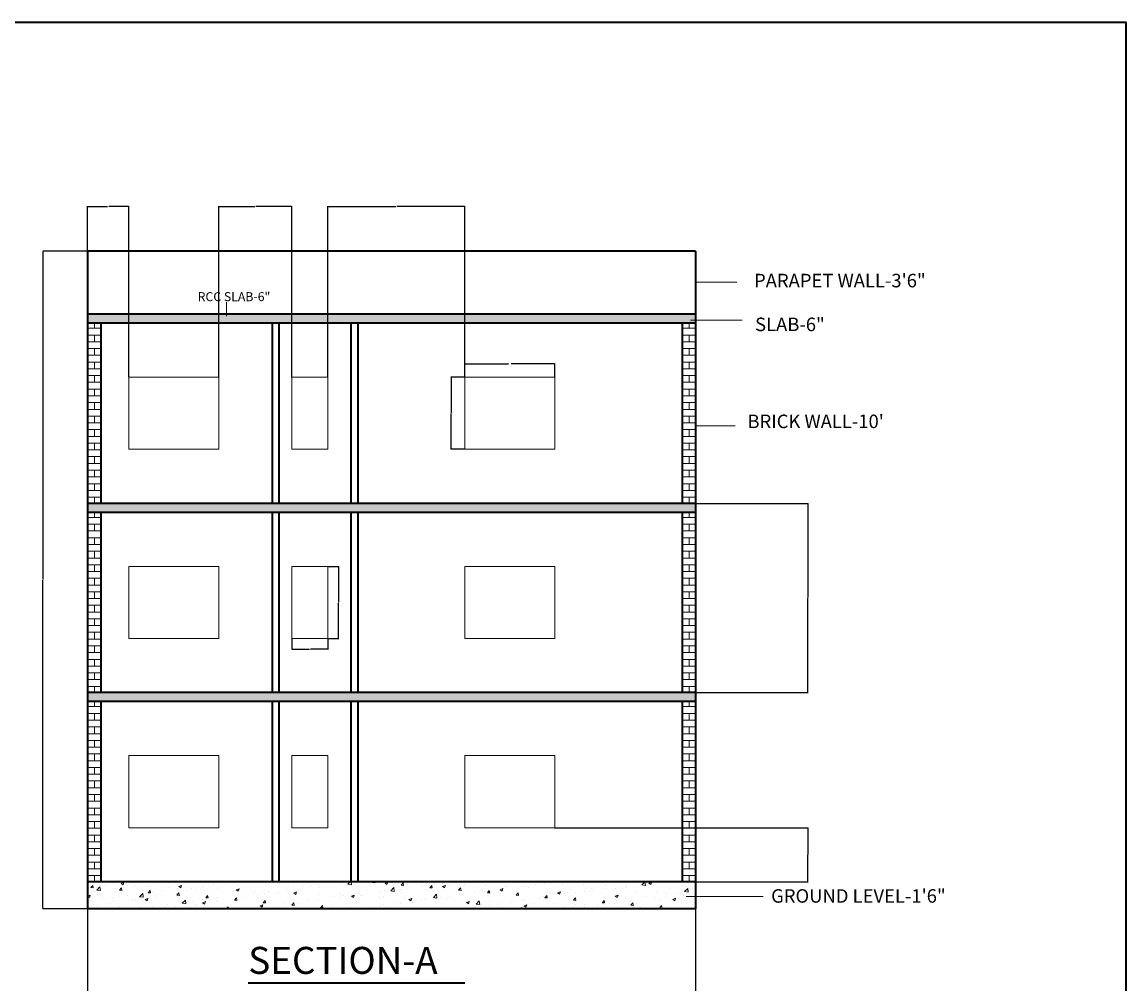
# Model space of a CAD drawing. Units: inches. Extents: x 1955 to 3324, y 980 to 3129.
# Tile 11 of 11: x 2589 to 3324, y 2488 to 3129. Entities that reach past the tile are written whole.
import ezdxf

# ---------------------------------------------------------------- set-up
doc = ezdxf.new("R2010")
doc.units = ezdxf.units.IN
for name, color, linetype, lineweight in [('A-ANNO-DIMS', 2, 'Continuous', 18), ('A-ANNO-TEXT', 7, 'Continuous', 18), ('A-ANNO-TITL', 7, 'Continuous', 35), ('A-ANNO-TTLB', 7, 'Continuous', 35), ('A-GLAZ', 4, 'Continuous', 18), ('A-SECT', 7, 'Continuous', 35), ('A-WALL-PATT', 252, 'Continuous', 13), ('S-CONC-PATT', 252, 'Continuous', 13), ('S-SLAB', 7, 'Continuous', 35)]:
    doc.layers.add(name, color=color, linetype=linetype, lineweight=lineweight)
doc.styles.get("Standard").update_dxf_attribs({"font": 'arial.ttf'})
doc.dimstyles.get("Standard").update_dxf_attribs({"dimtxt": 0.18, "dimasz": 0.18, "dimexe": 0.18, "dimexo": 0.0625, "dimgap": 0.09, "dimtad": 0, "dimtih": 1, "dimtoh": 1, "dimdec": 4, "dimzin": 0, "dimdsep": 46, "dimtxsty": 'Standard', "dimcen": 0.09, "dimadec": 0, "dimazin": 0, "dimtfac": 1, "dimtdec": 4, "dimtofl": 0, "dimtmove": 0, "dimatfit": 3, "dimfxl": 1, "dimtolj": 1, "dimtzin": 0, "dimarcsym": 0})

# ---------------------------------------------------------------- blocks, each defined once
blk = doc.blocks.new('WIN-SECT-60')
for p, q in [((0, 48), (0, 0)), ((60, 48), (0, 48)), ((60, 48), (60, 0)), ((60, 0), (0, 0))]:
    blk.add_line(p, q)
blk = doc.blocks.new('WIN-SECT-24')
for p, q in [((0, 48), (0, 0)), ((24, 48), (0, 48)), ((24, 48), (24, 0)), ((24, 0), (0, 0))]:
    blk.add_line(p, q)
blk = doc.blocks.new('*D47')
at = {"layer": 'A-ANNO-DIMS', "color": 0, "lineweight": -2, "transparency": 16777216}
for p, q in [((2883.64, 2892.47), (2883.64, 2901.59)), ((2883.82, 2901.41), (2912.79, 2901.41)), ((2943.46, 2901.41), (2914.48, 2901.41)), ((2943.64, 2892.47), (2943.64, 2901.59))]:
    blk.add_line(p, q, dxfattribs=at)
at = {"layer": 'A-ANNO-DIMS', "color": 0, "transparency": 16777216}
for points in [[(2883.82, 2901.44), (2883.82, 2901.38), (2883.64, 2901.41)], [(2943.46, 2901.44), (2943.46, 2901.38), (2943.64, 2901.41)]]:
    blk.add_solid(points, dxfattribs=at)
at = {"layer": 'Defpoints', "color": 0, "transparency": 16777216}
for p in [(2883.64, 2901.41), (2883.64, 2892.41), (2943.64, 2892.41)]:
    blk.add_point(p, dxfattribs=at)
at = {"layer": 'A-ANNO-DIMS', "color": 0, "transparency": 16777216, "insert": (2913.64, 2901.41), "char_height": 0.18, "attachment_point": 5}
blk.add_mtext('\\A1;WIN. 60 TYP.', dxfattribs=at)
blk = doc.blocks.new('*D48')
at = {"layer": 'A-ANNO-DIMS', "color": 0, "lineweight": -2, "transparency": 16777216}
for p, q in [((2883.57, 2892.41), (2874.46, 2892.41)), ((2874.64, 2892.23), (2874.64, 2868.59)), ((2874.64, 2844.59), (2874.64, 2868.23)), ((2883.57, 2844.41), (2874.46, 2844.41))]:
    blk.add_line(p, q, dxfattribs=at)
at = {"layer": 'A-ANNO-DIMS', "color": 0, "transparency": 16777216}
for points in [[(2874.61, 2892.23), (2874.67, 2892.23), (2874.64, 2892.41)], [(2874.61, 2844.59), (2874.67, 2844.59), (2874.64, 2844.41)]]:
    blk.add_solid(points, dxfattribs=at)
at = {"layer": 'Defpoints', "color": 0, "transparency": 16777216}
for p in [(2883.64, 2892.41), (2874.64, 2844.41), (2883.64, 2844.41)]:
    blk.add_point(p, dxfattribs=at)
at = {"layer": 'A-ANNO-DIMS', "color": 0, "transparency": 16777216, "insert": (2874.64, 2868.41), "char_height": 0.18, "attachment_point": 5}
blk.add_mtext('\\A1;48 TYP.', dxfattribs=at)
blk = doc.blocks.new('*D49')
at = {"layer": 'A-ANNO-DIMS', "color": 0, "lineweight": -2, "transparency": 16777216}
for p, q in [((2792.5, 2766.41), (2799.81, 2766.41)), ((2799.63, 2766.23), (2799.63, 2742.59)), ((2799.63, 2718.59), (2799.63, 2742.23)), ((2792.5, 2718.41), (2799.81, 2718.41))]:
    blk.add_line(p, q, dxfattribs=at)
at = {"layer": 'A-ANNO-DIMS', "color": 0, "transparency": 16777216}
for points in [[(2799.6, 2766.23), (2799.66, 2766.23), (2799.63, 2766.41)], [(2799.6, 2718.59), (2799.66, 2718.59), (2799.63, 2718.41)]]:
    blk.add_solid(points, dxfattribs=at)
at = {"layer": 'Defpoints', "color": 0, "transparency": 16777216}
for p in [(2792.43, 2766.41), (2799.63, 2766.41), (2792.43, 2718.41)]:
    blk.add_point(p, dxfattribs=at)
at = {"layer": 'A-ANNO-DIMS', "color": 0, "transparency": 16777216, "insert": (2799.63, 2742.41), "char_height": 0.18, "attachment_point": 5}
blk.add_mtext('\\A1;WIN. 48 TYP.', dxfattribs=at)
blk = doc.blocks.new('*D50')
at = {"layer": 'A-ANNO-DIMS', "color": 0, "lineweight": -2, "transparency": 16777216}
for p, q in [((2768.43, 2718.35), (2768.43, 2711.03)), ((2792.43, 2718.35), (2792.43, 2711.03)), ((2768.61, 2711.21), (2779.91, 2711.21)), ((2792.25, 2711.21), (2780.96, 2711.21))]:
    blk.add_line(p, q, dxfattribs=at)
at = {"layer": 'A-ANNO-DIMS', "color": 0, "transparency": 16777216}
for points in [[(2768.61, 2711.24), (2768.61, 2711.18), (2768.43, 2711.21)], [(2792.25, 2711.24), (2792.25, 2711.18), (2792.43, 2711.21)]]:
    blk.add_solid(points, dxfattribs=at)
at = {"layer": 'Defpoints', "color": 0, "transparency": 16777216}
for p in [(2768.43, 2718.41), (2792.43, 2718.41), (2792.43, 2711.21)]:
    blk.add_point(p, dxfattribs=at)
at = {"layer": 'A-ANNO-DIMS', "color": 0, "transparency": 16777216, "insert": (2780.43, 2711.21), "char_height": 0.18, "attachment_point": 5}
blk.add_mtext('\\A1;24 TYP.', dxfattribs=at)
blk = doc.blocks.new('*D132')
at = {"layer": 'A-ANNO-DIMS', "color": 0, "lineweight": -2, "transparency": 16777216}
for p, q in [((2632.37, 2538.35), (2632.37, 2459.05)), ((3037.37, 2538.35), (3037.37, 2459.05)), ((2632.55, 2459.23), (2834.58, 2459.23)), ((3037.19, 2459.23), (2835.16, 2459.23))]:
    blk.add_line(p, q, dxfattribs=at)
at = {"layer": 'A-ANNO-DIMS', "color": 0, "transparency": 16777216}
for points in [[(2632.55, 2459.26), (2632.55, 2459.2), (2632.37, 2459.23)], [(3037.19, 2459.26), (3037.19, 2459.2), (3037.37, 2459.23)]]:
    blk.add_solid(points, dxfattribs=at)
at = {"layer": 'Defpoints', "color": 0, "transparency": 16777216}
for p in [(2632.37, 2538.41), (3037.37, 2538.41), (3037.37, 2459.23)]:
    blk.add_point(p, dxfattribs=at)
at = {"layer": 'A-ANNO-DIMS', "color": 0, "transparency": 16777216, "insert": (2834.87, 2459.23), "char_height": 0.18, "attachment_point": 5}
blk.add_mtext('\\A1;405', dxfattribs=at)
blk = doc.blocks.new('*D133')
at = {"layer": 'A-ANNO-DIMS', "color": 0, "lineweight": -2, "transparency": 16777216}
for p, q in [((2632.31, 2976.41), (2602.54, 2976.41)), ((2602.72, 2976.23), (2602.72, 2757.59)), ((2602.72, 2538.59), (2602.72, 2757.23)), ((2632.31, 2538.41), (2602.54, 2538.41))]:
    blk.add_line(p, q, dxfattribs=at)
at = {"layer": 'A-ANNO-DIMS', "color": 0, "transparency": 16777216}
for points in [[(2602.69, 2976.23), (2602.75, 2976.23), (2602.72, 2976.41)], [(2602.69, 2538.59), (2602.75, 2538.59), (2602.72, 2538.41)]]:
    blk.add_solid(points, dxfattribs=at)
at = {"layer": 'Defpoints', "color": 0, "transparency": 16777216}
for p in [(2602.72, 2976.41), (2632.37, 2976.41), (2632.37, 2538.41)]:
    blk.add_point(p, dxfattribs=at)
at = {"layer": 'A-ANNO-DIMS', "color": 0, "transparency": 16777216, "insert": (2602.72, 2757.41), "char_height": 0.18, "attachment_point": 5}
blk.add_mtext('\\A1;438', dxfattribs=at)
blk = doc.blocks.new('*D134')
at = {"layer": 'A-ANNO-DIMS', "color": 0, "lineweight": -2, "transparency": 16777216}
for p, q in [((3037.43, 2808.41), (3112.24, 2808.41)), ((3112.06, 2808.23), (3112.06, 2745.59)), ((3112.06, 2682.59), (3112.06, 2745.23)), ((3037.43, 2682.41), (3112.24, 2682.41))]:
    blk.add_line(p, q, dxfattribs=at)
at = {"layer": 'A-ANNO-DIMS', "color": 0, "transparency": 16777216}
for points in [[(3112.03, 2808.23), (3112.09, 2808.23), (3112.06, 2808.41)], [(3112.03, 2682.59), (3112.09, 2682.59), (3112.06, 2682.41)]]:
    blk.add_solid(points, dxfattribs=at)
at = {"layer": 'Defpoints', "color": 0, "transparency": 16777216}
for p in [(3037.37, 2808.41), (3112.06, 2808.41), (3037.37, 2682.41)]:
    blk.add_point(p, dxfattribs=at)
at = {"layer": 'A-ANNO-DIMS', "color": 0, "transparency": 16777216, "insert": (3112.06, 2745.41), "char_height": 0.18, "attachment_point": 5}
blk.add_mtext('\\A1;126', dxfattribs=at)
blk = doc.blocks.new('*D135')
at = {"layer": 'A-ANNO-DIMS', "color": 0, "lineweight": -2, "transparency": 16777216}
for p, q in [((2943.7, 2592.41), (3112.24, 2592.41)), ((3112.06, 2592.23), (3112.06, 2574.59)), ((3112.06, 2556.59), (3112.06, 2574.23)), ((3028.43, 2556.41), (3112.24, 2556.41))]:
    blk.add_line(p, q, dxfattribs=at)
at = {"layer": 'A-ANNO-DIMS', "color": 0, "transparency": 16777216}
for points in [[(3112.03, 2592.23), (3112.09, 2592.23), (3112.06, 2592.41)], [(3112.03, 2556.59), (3112.09, 2556.59), (3112.06, 2556.41)]]:
    blk.add_solid(points, dxfattribs=at)
at = {"layer": 'Defpoints', "color": 0, "transparency": 16777216}
for p in [(2943.64, 2592.41), (3028.37, 2556.41), (3112.06, 2556.41)]:
    blk.add_point(p, dxfattribs=at)
at = {"layer": 'A-ANNO-DIMS', "color": 0, "transparency": 16777216, "insert": (3112.06, 2574.41), "char_height": 0.18, "attachment_point": 5}
blk.add_mtext('\\A1;36', dxfattribs=at)
blk = doc.blocks.new('*D136')
at = {"layer": 'A-ANNO-DIMS', "color": 0, "lineweight": -2, "transparency": 16777216}
for p, q in [((2632.37, 2976.47), (2632.37, 3006.24)), ((2632.55, 3006.06), (2645.71, 3006.06)), ((2659.66, 3006.06), (2646.5, 3006.06)), ((2659.84, 2892.47), (2659.84, 3006.24))]:
    blk.add_line(p, q, dxfattribs=at)
at = {"layer": 'A-ANNO-DIMS', "color": 0, "transparency": 16777216}
for points in [[(2632.55, 3006.09), (2632.55, 3006.03), (2632.37, 3006.06)], [(2659.66, 3006.09), (2659.66, 3006.03), (2659.84, 3006.06)]]:
    blk.add_solid(points, dxfattribs=at)
at = {"layer": 'Defpoints', "color": 0, "transparency": 16777216}
for p in [(2659.84, 3006.06), (2632.37, 2976.41), (2659.84, 2892.41)]:
    blk.add_point(p, dxfattribs=at)
at = {"layer": 'A-ANNO-DIMS', "color": 0, "transparency": 16777216, "insert": (2646.1, 3006.06), "char_height": 0.18, "attachment_point": 5}
blk.add_mtext('\\A1;27.47', dxfattribs=at)
blk = doc.blocks.new('*D137')
at = {"layer": 'A-ANNO-DIMS', "color": 0, "lineweight": -2, "transparency": 16777216}
for p, q in [((2719.84, 2892.47), (2719.84, 3006.24)), ((2720.02, 3006.06), (2743.74, 3006.06)), ((2768.25, 3006.06), (2744.53, 3006.06)), ((2768.43, 2892.47), (2768.43, 3006.24))]:
    blk.add_line(p, q, dxfattribs=at)
at = {"layer": 'A-ANNO-DIMS', "color": 0, "transparency": 16777216}
for points in [[(2720.02, 3006.09), (2720.02, 3006.03), (2719.84, 3006.06)], [(2768.25, 3006.09), (2768.25, 3006.03), (2768.43, 3006.06)]]:
    blk.add_solid(points, dxfattribs=at)
at = {"layer": 'Defpoints', "color": 0, "transparency": 16777216}
for p in [(2768.43, 3006.06), (2719.84, 2892.41), (2768.43, 2892.41)]:
    blk.add_point(p, dxfattribs=at)
at = {"layer": 'A-ANNO-DIMS', "color": 0, "transparency": 16777216, "insert": (2744.14, 3006.06), "char_height": 0.18, "attachment_point": 5}
blk.add_mtext('\\A1;48.59', dxfattribs=at)
blk = doc.blocks.new('*D138')
at = {"layer": 'A-ANNO-DIMS', "color": 0, "lineweight": -2, "transparency": 16777216}
for p, q in [((2792.43, 2892.47), (2792.43, 3006.24)), ((2792.61, 3006.06), (2837.71, 3006.06)), ((2883.46, 3006.06), (2838.36, 3006.06)), ((2883.64, 2892.47), (2883.64, 3006.24))]:
    blk.add_line(p, q, dxfattribs=at)
at = {"layer": 'A-ANNO-DIMS', "color": 0, "transparency": 16777216}
for points in [[(2792.61, 3006.09), (2792.61, 3006.03), (2792.43, 3006.06)], [(2883.46, 3006.09), (2883.46, 3006.03), (2883.64, 3006.06)]]:
    blk.add_solid(points, dxfattribs=at)
at = {"layer": 'Defpoints', "color": 0, "transparency": 16777216}
for p in [(2883.64, 3006.06), (2792.43, 2892.41), (2883.64, 2892.41)]:
    blk.add_point(p, dxfattribs=at)
at = {"layer": 'A-ANNO-DIMS', "color": 0, "transparency": 16777216, "insert": (2838.04, 3006.06), "char_height": 0.18, "attachment_point": 5}
blk.add_mtext('\\A1;91.2', dxfattribs=at)

msp = doc.modelspace()

# ---------------------------------------------------------------- hatches: boundary and pattern name
at = {"layer": 'A-WALL-PATT'}
h = msp.add_hatch(dxfattribs=at)
h.set_pattern_fill('ANSI32', color=256)
h.paths.add_polyline_path([(2361.4775, 2456.5037), (2270.2755, 2456.5037), (2270.2755, 2447.5037), (2285.7102, 2447.5037), (2285.7102, 2363.5037), (2281.1795, 2363.5037), (2281.1795, 2359.0037), (2290.2102, 2359.0037), (2290.2102, 2447.5037), (2361.4775, 2447.5037), (2361.4775, 2452.0037)])
h.paths.add_polyline_path([(2246.2755, 2456.5037), (2197.6809, 2456.5037), (2197.6809, 2447.5037), (2233.2102, 2447.5037), (2233.2102, 2355.6044), (2237.7102, 2355.6044), (2237.7102, 2447.5037), (2246.2755, 2447.5037)], flags=17)
h.paths.add_polyline_path([(2137.6809, 2456.5037), (2110.2102, 2456.5037), (2110.2102, 2312.5037), (2152.2102, 2312.5037), (2281.2102, 2312.5037), (2281.2102, 2107.6185), (2290.2102, 2107.6185), (2290.2102, 2267.9289), (2329.216, 2267.9289), (2329.216, 2272.4289), (2329.216, 2276.9289), (2290.2102, 2276.9289), (2290.2102, 2321.5037), (2281.2102, 2321.5037), (2119.2102, 2321.5037), (2119.2102, 2447.5037), (2137.6809, 2447.5037)])
h.paths.add_polyline_path([(2515.2102, 2456.5037), (2421.4775, 2456.5037), (2421.4775, 2447.5037), (2506.2102, 2447.5037), (2506.2102, 2415.6626), (2515.2102, 2415.6626)])
h.paths.add_polyline_path([(2515.2102, 2355.6626), (2506.2102, 2355.6626), (2506.2102, 2321.5037), (2424.9282, 2321.5037), (2424.9282, 2312.5037), (2461.2102, 2312.5037), (2470.2102, 2312.5037), (2515.2102, 2312.5037)])
h.paths.add_polyline_path([(2515.2102, 2232.5037), (2470.2102, 2232.5037), (2470.2102, 2237.3759), (2465.7102, 2237.3759), (2461.2102, 2237.3759), (2461.2102, 2232.5037), (2377.2219, 2232.5037), (2377.2219, 2321.5037), (2368.2219, 2321.5037), (2368.2219, 2276.9289), (2359.3802, 2276.9289), (2359.3802, 2272.4289), (2359.3802, 2267.9289), (2368.2219, 2267.9289), (2368.2219, 2223.5037), (2377.2219, 2223.5037), (2461.2102, 2223.5037), (2506.2102, 2223.5037), (2506.2102, 2129.5037), (2461.2102, 2129.5037), (2387.2102, 2129.5037), (2368.2219, 2129.5037), (2368.2219, 2056.4936), (2361.0095, 2056.4936), (2361.0095, 2051.9936), (2361.0095, 2047.4936), (2368.2219, 2047.4936), (2368.2219, 2031.5037), (2377.2219, 2031.5037), (2377.2219, 2120.5037), (2461.2102, 2120.5037), (2461.2102, 2112.7921), (2470.2102, 2112.7921), (2470.2102, 2120.5037), (2515.2102, 2120.5037), (2515.2102, 2129.5037)])
h.paths.add_polyline_path([(2470.2102, 2277.1758), (2461.2102, 2277.1758), (2461.2102, 2272.5037), (2461.2102, 2270.2549), (2470.2102, 2270.2549), (2470.2102, 2272.5037)], flags=17)
h.paths.add_polyline_path([(2515.2102, 2040.5037), (2470.2102, 2040.5037), (2417.8264, 2040.5037), (2417.8264, 2031.5037), (2506.2102, 2031.5037), (2506.2102, 2005.3639), (2515.2102, 2005.3639)])
h.paths.add_polyline_path([(2506.2102, 1905.5037), (2402.6963, 1905.5037), (2402.6963, 1896.5037), (2506.2102, 1896.5037)])
h.paths.add_polyline_path([(2515.2102, 1945.3639), (2506.2102, 1945.3639), (2506.2102, 1905.5037), (2506.2102, 1896.5037), (2515.2102, 1896.5037)])
h.paths.add_polyline_path([(2342.6963, 1901.0037), (2342.6963, 1905.5037), (2273.4892, 1905.5037), (2273.4892, 1896.5037), (2342.6963, 1896.5037)])
h.paths.add_polyline_path([(2290.2102, 1994.0037), (2283.612, 1994.0037), (2283.612, 1991.7537), (2283.612, 1989.5037), (2285.7102, 1989.5037), (2285.7102, 1905.5037), (2290.2102, 1905.5037)])
h.paths.add_polyline_path([(2249.4892, 1905.5037), (2237.7102, 1905.5037), (2206.3617, 1905.5037), (2206.3617, 1896.5037), (2249.4892, 1896.5037), (2249.4892, 1901.0037)])
h.paths.add_polyline_path([(2237.7102, 1989.5037), (2261.7102, 1989.5037), (2261.7102, 1994.0037), (2237.7102, 1994.0037), (2237.7102, 1999.266), (2235.4602, 1999.266), (2233.2102, 1999.266), (2233.2102, 1994.0037), (2233.2102, 1905.5037), (2237.7102, 1905.5037)])
h.paths.add_polyline_path([(2119.2102, 1947.5144), (2110.2102, 1947.5144), (2110.2102, 1896.5037), (2119.2102, 1896.5037), (2146.3617, 1896.5037), (2146.3617, 1901.0037), (2146.3617, 1905.5037), (2119.2102, 1905.5037)])
h.paths.add_polyline_path([(2119.2102, 2068.6379), (2110.2102, 2068.6379), (2110.2102, 2007.5144), (2119.2102, 2007.5144), (2119.2102, 2031.5037), (2233.2102, 2031.5037), (2233.2102, 2027.9287), (2235.4602, 2027.9287), (2237.7102, 2027.9287), (2237.7102, 2031.5037), (2281.2102, 2031.5037), (2290.2102, 2031.5037), (2290.2102, 2047.4936), (2326.409, 2047.4936), (2326.409, 2056.4936), (2290.2102, 2056.4936), (2290.2102, 2071.2722), (2285.7102, 2071.2722), (2281.2102, 2071.2722), (2281.2102, 2040.5037), (2227.2102, 2040.5037), (2227.2102, 2111.2571), (2222.7102, 2111.2571), (2218.2102, 2111.2571), (2218.2102, 2040.5037), (2119.2102, 2040.5037)])
h.paths.add_polyline_path([(2236.9166, 2214.5037), (2161.2102, 2214.5037), (2161.2102, 2221.6488), (2152.2102, 2221.6488), (2152.2102, 2214.5037), (2110.2102, 2214.5037), (2110.2102, 2205.5037), (2131.2394, 2205.5037), (2131.2394, 2198.3478), (2140.2394, 2198.3478), (2140.2394, 2205.5037), (2224.2394, 2205.5037), (2224.2394, 2200.2317), (2228.7394, 2200.2317), (2233.2394, 2200.2317), (2233.2394, 2205.5037), (2236.9166, 2205.5037)], flags=17)
h.paths.add_polyline_path([(2236.9166, 2157.5037), (2233.2394, 2157.5037), (2233.2394, 2178.9172), (2228.7394, 2178.9172), (2224.2394, 2178.9172), (2224.2394, 2157.5037), (2140.2394, 2157.5037), (2140.2394, 2174.3478), (2131.2394, 2174.3478), (2131.2394, 2157.5037), (2110.2102, 2157.5037), (2110.2102, 2128.6379), (2119.2102, 2128.6379), (2119.2102, 2148.5037), (2218.2102, 2148.5037), (2218.2102, 2141.7262), (2222.7102, 2141.7262), (2227.2102, 2141.7262), (2227.2102, 2148.5037), (2236.9166, 2148.5037)], flags=0)
h.paths.add_polyline_path([(3084.7449, 2537.3808), (3212.7954, 2537.3808), (3212.7954, 2555.9271), (3084.7449, 2555.9271)], flags=9)
h.paths.add_polyline_path([(3068.7485, 2853.43), (3169.977, 2853.43), (3169.977, 2871.9764), (3068.7485, 2871.9764)], flags=9)
h.paths.add_polyline_path([(3074.1798, 2918.0252), (3126.4732, 2918.0252), (3126.4732, 2936.5716), (3074.1798, 2936.5716)], flags=9)
h.paths.add_polyline_path([(3073.0928, 2947.3127), (3199.0499, 2947.3127), (3199.0499, 2965.8591), (3073.0928, 2965.8591)], flags=9)
h.paths.add_polyline_path([(2733.8393, 2484.8678), (2879.7915, 2484.8678), (2879.7915, 2521.9606), (2733.8393, 2521.9606)], flags=9)
h.paths.add_polyline_path([(2204.9881, 2482.4168), (2355.1272, 2482.4168), (2355.1272, 2519.5095), (2204.9881, 2519.5095)], flags=9)
h.paths.add_polyline_path([(3062.1429, 2387.2466), (3079.3735, 2387.2466), (3079.3735, 2411.9751), (3062.1429, 2411.9751)], flags=9)
h.paths.add_polyline_path([(2190.1574, 2158.8439), (2219.315, 2158.8439), (2219.315, 2177.5013), (2190.1574, 2177.5013)], flags=25)
h.paths.add_polyline_path([(2213.6766, 1840.7276), (2405.0382, 1840.7276), (2405.0382, 1865.4561), (2213.6766, 1865.4561)], flags=9)
h.paths.add_polyline_path([(2180.5398, 2233.911), (2213.9471, 2233.911), (2213.9471, 2252.5683), (2180.5398, 2252.5683)], flags=25)
h.paths.add_polyline_path([(2134.4484, 2238.3973), (2134.4484, 2274.2807), (2115.791, 2274.2807), (2115.791, 2238.3973)], flags=25)
h.paths.add_polyline_path([(2135.1593, 2122.9991), (2173.7507, 2122.9991), (2173.7507, 2141.6565), (2135.1593, 2141.6565)], flags=25)
h.paths.add_polyline_path([(2129.8822, 2002.1912), (2168.4736, 2002.1912), (2168.4736, 2020.8486), (2129.8822, 2020.8486)], flags=9)
h.paths.add_polyline_path([(2239.6647, 1953.4107), (2268.8973, 1953.4107), (2268.8973, 1972.068), (2239.6647, 1972.068)], flags=9)
h.paths.add_polyline_path([(2352.8562, 1951.2904), (2402.1775, 1951.2904), (2402.1775, 1969.9477), (2352.8562, 1969.9477)], flags=9)
h.paths.add_polyline_path([(2500.1358, 2055.32), (2500.1358, 2091.2034), (2481.4784, 2091.2034), (2481.4784, 2055.32)], flags=25)
h.paths.add_polyline_path([(2391.2702, 2058.6821), (2424.4285, 2058.6821), (2424.4285, 2077.3394), (2391.2702, 2077.3394)], flags=25)
h.paths.add_polyline_path([(2507.7996, 2257.2758), (2507.7996, 2293.1592), (2489.1422, 2293.1592), (2489.1422, 2257.2758)], flags=25)
h.paths.add_polyline_path([(2386.8349, 2273.8734), (2419.9931, 2273.8734), (2419.9931, 2292.5307), (2386.8349, 2292.5307)], flags=25)
h.paths.add_polyline_path([(2335.374, 2373.3267), (2384.6953, 2373.3267), (2384.6953, 2391.984), (2335.374, 2391.984)], flags=9)
h.paths.add_polyline_path([(2243.8205, 2380.6539), (2273.0531, 2380.6539), (2273.0531, 2399.3113), (2243.8205, 2399.3113)], flags=25)
h.paths.add_polyline_path([(2126.2627, 2321.6894), (2164.8541, 2321.6894), (2164.8541, 2340.3467), (2126.2627, 2340.3467)], flags=25)
h = msp.add_hatch(dxfattribs=at)
h.set_pattern_fill('BRICK', color=256, scale=0.708661, style=0)
h.paths.add_polyline_path([(2632.3694, 2808.4103), (2641.3694, 2808.4103), (2641.3694, 2928.4103), (2632.3694, 2928.4103)])
h = msp.add_hatch(dxfattribs=at)
h.set_pattern_fill('BRICK', color=256, scale=0.708661, style=0)
h.paths.add_polyline_path([(3028.3694, 2808.4103), (3037.3694, 2808.4103), (3037.3694, 2928.4103), (3028.3694, 2928.4103)])
h = msp.add_hatch(dxfattribs=at)
h.set_pattern_fill('BRICK', color=256, scale=0.708661, style=0)
h.paths.add_polyline_path([(2632.3694, 2682.4103), (2641.3694, 2682.4103), (2641.3694, 2802.4103), (2632.3694, 2802.4103)])
h = msp.add_hatch(dxfattribs=at)
h.set_pattern_fill('BRICK', color=256, scale=0.708661, style=0)
h.paths.add_polyline_path([(3028.3694, 2682.4103), (3037.3694, 2682.4103), (3037.3694, 2802.4103), (3028.3694, 2802.4103)])
h = msp.add_hatch(dxfattribs=at)
h.set_pattern_fill('BRICK', color=256, scale=0.708661, style=0)
h.paths.add_polyline_path([(2632.3694, 2556.4103), (2641.3694, 2556.4103), (2641.3694, 2676.4103), (2632.3694, 2676.4103)])
h = msp.add_hatch(dxfattribs=at)
h.set_pattern_fill('BRICK', color=256, scale=0.708661, style=0)
h.paths.add_polyline_path([(3028.3694, 2556.4103), (3037.3694, 2556.4103), (3037.3694, 2676.4103), (3028.3694, 2676.4103)])
at = {"layer": 'S-CONC-PATT'}
h = msp.add_hatch(dxfattribs=at)
h.set_pattern_fill('AR-CONC', color=256, scale=0.052, style=0)
h.paths.add_polyline_path([(2632.3694, 2928.4103), (3037.3694, 2928.4103), (3037.3694, 2934.4103), (2632.3694, 2934.4103)])
h = msp.add_hatch(dxfattribs=at)
h.set_pattern_fill('AR-CONC', color=256, scale=0.052, style=0)
h.paths.add_polyline_path([(2632.3694, 2802.4103), (3037.3694, 2802.4103), (3037.3694, 2808.4103), (2632.3694, 2808.4103)])
h = msp.add_hatch(dxfattribs=at)
h.set_pattern_fill('AR-CONC', color=256, scale=0.052, style=0)
h.paths.add_polyline_path([(2632.3694, 2676.4103), (3037.3694, 2676.4103), (3037.3694, 2682.4103), (2632.3694, 2682.4103)])
h = msp.add_hatch(dxfattribs=at)
h.set_pattern_fill('AR-CONC', color=256, scale=0.105, style=0)
h.paths.add_polyline_path([(2632.3694, 2538.4103), (3037.3694, 2538.4103), (3037.3694, 2556.4103), (2632.3694, 2556.4103)])

# ---------------------------------------------------------------- linework, layer by layer
at = {"layer": 'A-ANNO-TEXT'}
for p, q in [((3037.3694, 2955.6893), (3064.8388, 2955.6893)), ((2724.8869, 2932.9937), (2724.8869, 2942.3403)), ((3033.9245, 2930.4418), (3068.4187, 2930.4418)), ((3037.3694, 2860.0421), (3063.7764, 2860.0421)), ((3031.0747, 2546.554), (3082.4075, 2546.554))]:
    msp.add_line(p, q, dxfattribs=at)
at = {"layer": 'A-ANNO-TITL'}
msp.add_line((2883.801, 2488.8753), (2739.4689, 2488.8753), dxfattribs=at)
at = {"layer": 'A-ANNO-TTLB'}
msp.add_lwpolyline([(1954.5391, 3128.9103), (3323.9705, 3128.9103), (3323.9705, 1703.6826), (1954.5391, 1703.6826)], close=True, dxfattribs=at)
at = {"layer": 'A-SECT'}
for p, q in [((2632.3694, 2976.4103), (2632.3694, 2790.4103)), ((3037.3694, 2976.4103), (2632.3694, 2976.4103)), ((3037.3694, 2976.4103), (3037.3694, 2790.4103)), ((2641.3694, 2928.4103), (2641.3694, 2808.4103)), ((2755.3694, 2928.4103), (2755.3694, 2808.4103)), ((2759.8694, 2928.4103), (2759.8694, 2808.4103)), ((2807.8694, 2928.4103), (2807.8694, 2808.4103)), ((2812.3694, 2928.4103), (2812.3694, 2808.4103)), ((3028.3694, 2928.4103), (3028.3694, 2808.4103)), ((2632.3694, 2850.4103), (2632.3694, 2664.4103)), ((3037.3694, 2850.4103), (3037.3694, 2664.4103)), ((2641.3694, 2802.4103), (2641.3694, 2682.4103)), ((2755.3694, 2802.4103), (2755.3694, 2682.4103)), ((2759.8694, 2802.4103), (2759.8694, 2682.4103)), ((2807.8694, 2802.4103), (2807.8694, 2682.4103)), ((2812.3694, 2802.4103), (2812.3694, 2682.4103)), ((3028.3694, 2802.4103), (3028.3694, 2682.4103)), ((2632.3694, 2724.4103), (2632.3694, 2538.4103)), ((3037.3694, 2724.4103), (3037.3694, 2538.4103)), ((2641.3694, 2676.4103), (2641.3694, 2556.4103)), ((2755.3694, 2676.4103), (2755.3694, 2556.4103)), ((2759.8694, 2676.4103), (2759.8694, 2556.4103)), ((2807.8694, 2676.4103), (2807.8694, 2556.4103)), ((2812.3694, 2676.4103), (2812.3694, 2556.4103)), ((3028.3694, 2676.4103), (3028.3694, 2556.4103))]:
    msp.add_line(p, q, dxfattribs=at)
at = {"layer": 'S-SLAB'}
for p, q in [((3037.3694, 2934.4103), (2632.3694, 2934.4103)), ((3037.3694, 2928.4103), (2632.3694, 2928.4103)), ((3037.3694, 2808.4103), (2632.3694, 2808.4103)), ((3037.3694, 2802.4103), (2632.3694, 2802.4103)), ((3037.3694, 2682.4103), (2632.3694, 2682.4103)), ((3037.3694, 2676.4103), (2632.3694, 2676.4103)), ((3037.3694, 2556.4103), (2632.3694, 2556.4103)), ((3037.3694, 2538.4103), (2632.3694, 2538.4103))]:
    msp.add_line(p, q, dxfattribs=at)

# ---------------------------------------------------------------- block references
at = {"layer": 'A-GLAZ', "rotation": 180}
for p in [(2719.84, 2892.4106), (2943.6367, 2892.4106), (2719.84, 2766.4106), (2943.6367, 2766.4106), (2943.6367, 2640.4106)]:
    msp.add_blockref('WIN-SECT-60', p, dxfattribs=at)
at = {"layer": 'A-GLAZ'}
for name, p in [('WIN-SECT-24', (2768.435, 2844.41)), ('WIN-SECT-24', (2768.435, 2718.41)), ('WIN-SECT-60', (2659.84, 2592.41)), ('WIN-SECT-24', (2768.435, 2592.41))]:
    msp.add_blockref(name, p, dxfattribs=at)

# ---------------------------------------------------------------- texts
at = {"layer": 'A-ANNO-TEXT', "attachment_point": 1}
for s, width, insert, char_height in [('PARAPET WALL-3\'6"', 289.957819, (3076.3128, 2961.2639), 9), ('RCC SLAB-6"', 70.859128, (2705.7465, 2949.0426), 6), ('SLAB-6"', 64.53499, (3076.9946, 2932.0931), 9), ("BRICK WALL-10'", 167.383059, (3071.9194, 2867.4979), 9), ('GROUND LEVEL-1\'6"', 194.2928, (3087.6641, 2551.4548), 9)]:
    msp.add_mtext_dynamic_manual_height_columns(s, width=width, gutter_width=12.5, heights=[0], dxfattribs=dict(at, insert=insert, char_height=char_height))
at = {"layer": 'A-ANNO-TITL', "insert": (2739.4689, 2513.0159), "char_height": 18, "attachment_point": 1}
msp.add_mtext_dynamic_manual_height_columns('SECTION-A', width=250.434392, gutter_width=12.5, heights=[0], dxfattribs=at)

# ---------------------------------------------------------------- dimensions: what is measured, and where the dimension line sits
at = {"layer": 'A-ANNO-DIMS'}
for base, p1, p2, override, picture, middle in [((2659.84, 3006.0603), (2632.3694, 2976.4103), (2659.84, 2892.4103), {"dimdec": 2, "dimlfac": 1, "dimrnd": 0, "dimzin": 0, "dimdsep": 46, "dimlunit": 2}, '*D136', (2646.1047, 3006.0603)), ((2768.4346, 3006.0603), (2719.84, 2892.4103), (2768.4346, 2892.4103), {"dimdec": 2, "dimlfac": 1, "dimrnd": 0, "dimzin": 0, "dimdsep": 46, "dimlunit": 2}, '*D137', (2744.1373, 3006.0603)), ((2883.6367, 3006.0603), (2792.4346, 2892.4103), (2883.6367, 2892.4103), {"dimdec": 1, "dimlfac": 1, "dimrnd": 0, "dimzin": 0, "dimdsep": 46, "dimlunit": 2}, '*D138', (2838.0356, 3006.0603)), ((3037.3694, 2459.2253), (2632.3694, 2538.4103), (3037.3694, 2538.4103), {"dimdec": 0, "dimlfac": 1, "dimrnd": 0, "dimzin": 0, "dimdsep": 46, "dimlunit": 2}, '*D132', (2834.8694, 2459.2253))]:
    dim = msp.add_linear_dim(base=base, p1=p1, p2=p2, dimstyle='Standard', override=override, dxfattribs=at)
    dim.commit()
    dim.dimension.update_dxf_attribs({"geometry": picture, "text_midpoint": middle})
for base, p1, p2, picture, middle in [((2602.7194, 2976.4103), (2632.3694, 2538.4103), (2632.3694, 2976.4103), '*D133', (2602.7194, 2757.4103)), ((3112.0575, 2808.4103), (3037.3694, 2682.4103), (3037.3694, 2808.4103), '*D134', (3112.0575, 2745.4103)), ((3112.0575, 2556.4103), (2943.6367, 2592.4103), (3028.3694, 2556.4103), '*D135', (3112.0575, 2574.4103))]:
    dim = msp.add_linear_dim(base=base, p1=p1, p2=p2, angle=90, dimstyle='Standard', override={"dimdec": 0, "dimlfac": 1, "dimrnd": 0, "dimzin": 0, "dimdsep": 46, "dimlunit": 2}, dxfattribs=at)
    dim.commit()
    dim.dimension.update_dxf_attribs({"geometry": picture, "text_midpoint": middle})
for base, p1, p2, angle, text, picture, middle in [((2883.6367, 2901.4103), (2943.6367, 2892.4103), (2883.6367, 2892.4103), 180, 'WIN. <> TYP.', '*D47', (2913.6367, 2901.4103)), ((2874.6367, 2844.4103), (2883.6367, 2892.4103), (2883.6367, 2844.4103), 270, '<> TYP.', '*D48', (2874.6367, 2868.4103)), ((2799.6346, 2766.4103), (2792.4346, 2718.4103), (2792.4346, 2766.4103), 90, 'WIN. <> TYP.', '*D49', (2799.6346, 2742.4103))]:
    dim = msp.add_linear_dim(base=base, p1=p1, p2=p2, angle=angle, text=text, dimstyle='Standard', override={"dimdec": 0, "dimlfac": 1, "dimrnd": 0, "dimzin": 0, "dimdsep": 46, "dimlunit": 2}, dxfattribs=at)
    dim.commit()
    dim.dimension.update_dxf_attribs({"geometry": picture, "text_midpoint": middle})
dim = msp.add_linear_dim(base=(2792.4346, 2711.2103), p1=(2768.4346, 2718.4103), p2=(2792.4346, 2718.4103), text='<> TYP.', dimstyle='Standard', override={"dimdec": 0, "dimlfac": 1, "dimrnd": 0, "dimzin": 0, "dimdsep": 46, "dimlunit": 2}, dxfattribs=at)
dim.commit()
dim.dimension.update_dxf_attribs({"geometry": '*D50', "text_midpoint": (2780.4346, 2711.2103)})

doc.saveas('drawing.dxf')
